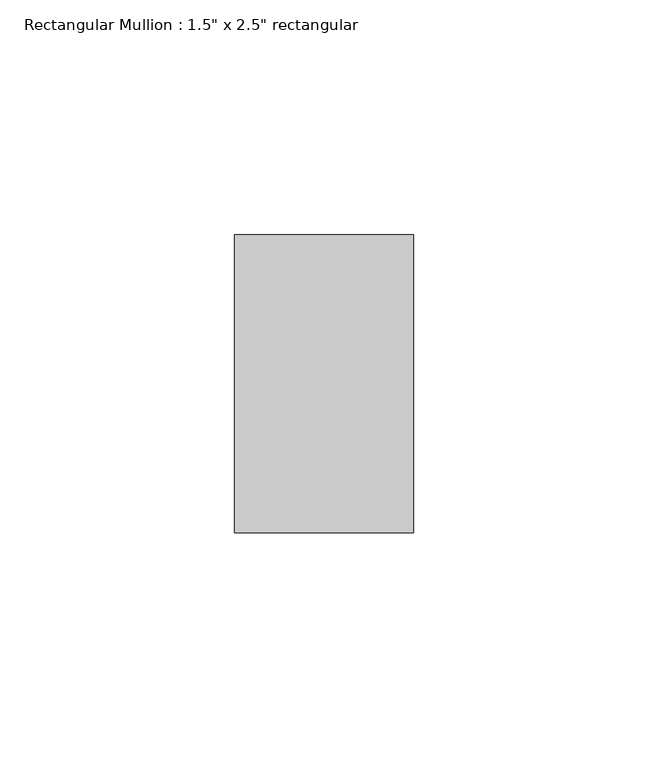
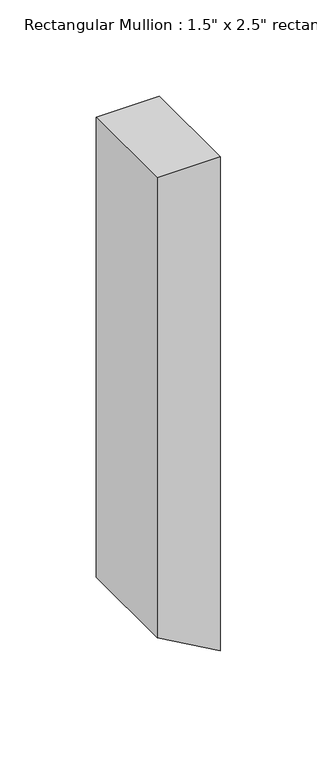
"""IFC4 building model written with IfcOpenShell, lengths in millimetres: member geometry."""

from ifc_helpers import new_model, si_unit, frame, origin, place, context, project, spatial, polyline, outline, extrude, source, transform, mapped, element, save


def member_f89b2291(model_context):
    return source(origin(), model_context, "Body", "SweptSolid", [
        extrude(outline(polyline([(0.0, 0.0), (0.0, -38.1), (-292.3156946, -38.1), (-313.9925526, 0.0), (0.0, 0.0)])), frame((0.0, -31.75, 0.0), z_axis=(0.0, 1.0, 0.0), x_axis=(0.0, 0.0, 1.0)), (0.0, 0.0, 1.0), 63.5),
    ])


if __name__ == "__main__":
    model = new_model("IFC4")
    model_context = context("Model", 3, world=origin())
    ifc_project = project(units=[si_unit("LENGTHUNIT", "METRE", prefix="MILLI")], contexts=[model_context])
    site = spatial("IfcSite", under=ifc_project)
    building = spatial("IfcBuilding", under=site)
    placement = place(None, origin())
    member_shape = member_f89b2291(model_context)
    element("IfcMember", 1, ObjectType="Rectangular Mullion : 1.5\" x 2.5\" rectangular", at=placement, inside=building, context=model_context, shape_type="MappedRepresentation", body=[
        mapped(member_shape, transform((0.0, 0.0, 0.0), x_axis=(1.0, 0.0, 0.0), y_axis=(0.0, 1.0, 0.0), z_axis=(0.0, 0.0, 1.0))),
    ])
    save(model, "model.ifc")

# Revit data of these elements
# Type "Rectangular Mullion : 1.5\" x 2.5\" rectangular"
#   built-in parameter 1007304 = 0.208333 (stored number, unit not read)
#   built-in parameter 1007301 = 0.0625 (stored number, unit not read)
#   built-in parameter 1007300 = 0.0625 (stored number, unit not read)
